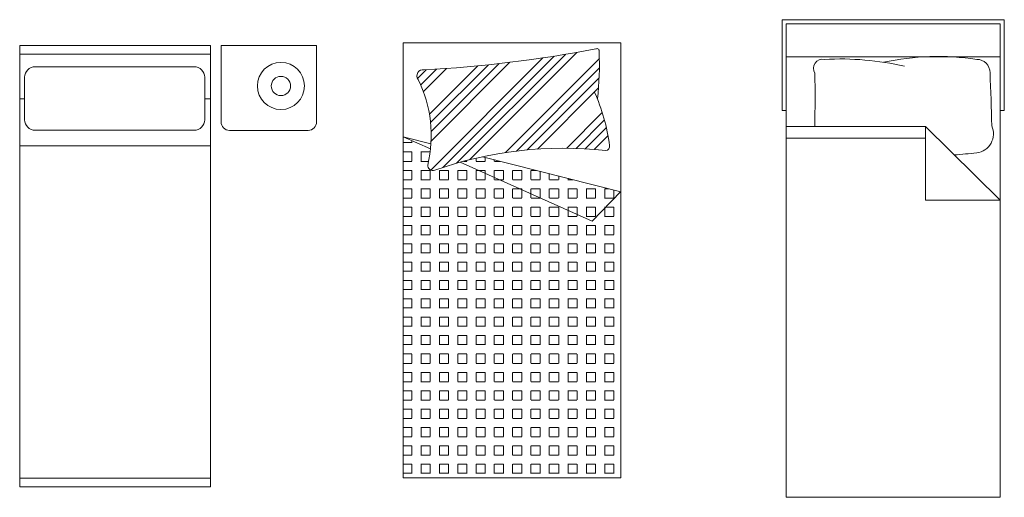
# Model space of a CAD drawing. Units: inches. Extents: x 1994 to 3075, y 3517 to 3950.
# Tile 4 of 58: x 1993.9156 to 1994.0985, y 3553.425 to 3553.5137. Entities that reach past the tile are written whole.
import ezdxf

# ---------------------------------------------------------------- set-up
doc = ezdxf.new("R2010")
doc.units = ezdxf.units.IN
doc.layers.add('A-FURN-REFR', color=8, linetype='Continuous', lineweight=13)
doc.layers.add('A-FURN-REFR-PATT', color=8, linetype='Continuous', lineweight=13)

msp = doc.modelspace()

# ---------------------------------------------------------------- hatches: boundary and pattern name
at = {"layer": 'A-FURN-REFR-PATT'}
h = msp.add_hatch(dxfattribs=at)
h.set_pattern_fill('ANSI34', color=256, scale=0.0003937007874016, style=0)
h.set_pattern_definition([(45, (1992.421944108623, 3552.870363246412), (-0.0053033008588991, 0.0053033008588991), []), (45, (1992.423711876339, 3552.870363246412), (-0.0053033008588991, 0.0053033008588991), []), (45, (1992.425479644056, 3552.870363246412), (-0.0053033008588991, 0.0053033008588991), []), (45, (1992.427247415709, 3552.870363246412), (-0.0053033008588991, 0.0053033008588991), [])])
h.paths.add_polyline_path([(1993.990115995337, 3553.504312261099, 0.3906811292884666), (1993.989395701099, 3553.503028519263, -0.1786183787400851), (1993.991383087467, 3553.486689302322, 0.5331944561183694), (1993.992669435749, 3553.485725398598, -0.1138350908180215), (1994.024455140842, 3553.489361875478, 0.4018271308504459), (1994.025167534964, 3553.490310392768, 0.0637529022039059), (1994.022888106701, 3553.498966425117, 0.0441980254026644), (1994.023194065573, 3553.508103659458, 0.2060157581720081), (1994.022937858968, 3553.508291233899, -0.033478375592124)])
h = msp.add_hatch(dxfattribs=at)
h.set_pattern_fill('SQUARE', color=256, scale=0.0005368647100931, style=0)
h.set_pattern_definition([(0, (1992.421944108623, 3552.870363246412), (0, 0.0017045454545455), [0.0017045454545455, -0.0017045454545455]), (90, (1992.421944108623, 3552.870363246412), (-0.0017045454545455, 0), [0.0017045454545455, -0.0017045454545455])])
h.paths.add_polyline_path([(1993.986843200924, 3553.428606654402), (1994.02722811466, 3553.428606654402), (1994.02722811466, 3553.481750477539), (1994.021907523152, 3553.476285841424), (1993.997414437724, 3553.487222591514, 0.0174826565834199), (1993.992669435749, 3553.485725398598, -0.5987234967258536), (1993.991383087467, 3553.486689302322, 0.0320212471709692), (1993.991893053683, 3553.489688021914), (1993.986843200924, 3553.491942902287)])
h.paths.add_polyline_path([(1994.00153542735, 3553.488234848997, 0.0149090101017854), (1993.997414437724, 3553.487222591514), (1994.021907523152, 3553.476285841424), (1994.02722811466, 3553.481750477539)], flags=17)

# ---------------------------------------------------------------- linework, layer by layer
at = {"layer": 'A-FURN-REFR'}
for p, q in [((1994.057231186005, 3553.496793440019), (1994.057231186005, 3553.513668440019)), ((1994.057231186005, 3553.513668440019), (1994.098481186005, 3553.513668440019)), ((1994.057981186005, 3553.51291844002), (1994.097731186004, 3553.51291844002)), ((1994.057981186005, 3553.51291844002), (1994.057981186005, 3553.496793440019)), ((1994.097731186004, 3553.51291844002), (1994.097731186004, 3553.496793440019)), ((1994.098481186005, 3553.513668440019), (1994.098481186005, 3553.496793440019)), ((1993.915581776324, 3553.426961523701), (1993.915581776324, 3553.508851287482)), ((1993.95101484719, 3553.508851287482), (1993.915581776324, 3553.508851287482)), ((1993.95101484719, 3553.426961523701), (1993.95101484719, 3553.508851287482)), ((1993.970718731013, 3553.508851287482), (1993.95300219558, 3553.508851287482)), ((1993.95300219558, 3553.508851287482), (1993.95300219558, 3553.494695899094)), ((1993.970718731013, 3553.494695899094), (1993.970718731013, 3553.508851287482)), ((1993.986843200924, 3553.509376481874), (1993.986843200924, 3553.428606654402)), ((1994.02722811466, 3553.509376481874), (1993.986843200924, 3553.509376481874)), ((1994.02722811466, 3553.509376481874), (1993.986843200924, 3553.509376481874)), ((1993.986843200924, 3553.509376481874), (1993.986843200924, 3553.428606654402)), ((1994.02722811466, 3553.493931850356), (1994.02722811466, 3553.509376481874)), ((1993.95101484719, 3553.507276484332), (1993.915581776324, 3553.507276484332)), ((1994.057981186005, 3553.425015883731), (1994.057981186005, 3553.50679344002)), ((1994.057981186005, 3553.50679344002), (1994.097731186004, 3553.50679344002)), ((1994.097731186004, 3553.50679344002), (1994.097731186004, 3553.425015883731)), ((1993.947992092256, 3553.504945443419), (1993.918464533201, 3553.504945443419)), ((1993.916496029264, 3553.502976939482), (1993.916496029264, 3553.495102923733)), ((1993.949960596193, 3553.495102923733), (1993.949960596193, 3553.502976939482)), ((1993.915581776324, 3553.498983996079), (1993.916496029264, 3553.498983996079)), ((1993.949960596193, 3553.498983996079), (1993.95101484719, 3553.498983996079)), ((1994.057981186005, 3553.496793440019), (1994.057231186005, 3553.496793440019)), ((1994.098481186005, 3553.496793440019), (1994.097731186004, 3553.496793440019)), ((1993.918464533201, 3553.493134419797), (1993.947992092256, 3553.493134419797)), ((1993.954576998729, 3553.493121095944), (1993.969143927863, 3553.493121095944)), ((1994.02722811466, 3553.428606654402), (1994.02722811466, 3553.493931850356)), ((1994.02722811466, 3553.428606654402), (1994.02722811466, 3553.493931850356)), ((1994.057982386004, 3553.49383344002), (1994.083847686004, 3553.49383344002)), ((1994.083847686004, 3553.49383344002), (1994.083847686004, 3553.48015344002)), ((1994.097732686005, 3553.48015344002), (1994.083847686004, 3553.49383344002)), ((1993.986843200924, 3553.491942902287), (1993.991974039738, 3553.490647970996)), ((1993.986843200924, 3553.491942902287), (1993.991893053683, 3553.489688021914)), ((1994.083847686004, 3553.49167344002), (1994.057982386004, 3553.49167344002)), ((1993.95101484719, 3553.490280994245), (1993.915581776324, 3553.490280994245)), ((1993.997414437724, 3553.487222591514), (1994.021907523152, 3553.476285841424)), ((1994.00153542735, 3553.488234848997), (1994.027238969916, 3553.481747737869)), ((1994.021907523152, 3553.476285841424), (1994.02722811466, 3553.481750477539)), ((1994.083847686004, 3553.48015344002), (1994.097732686005, 3553.48015344002)), ((1993.915581776324, 3553.428536326852), (1993.95101484719, 3553.428536326852)), ((1993.986843200924, 3553.428606654402), (1994.02722811466, 3553.428606654402)), ((1993.986843200924, 3553.428606654402), (1994.02722811466, 3553.428606654402)), ((1993.915581776324, 3553.426961523701), (1993.95101484719, 3553.426961523701)), ((1994.097731186004, 3553.425015883731), (1994.057981186005, 3553.425015883731))]:
    msp.add_line(p, q, dxfattribs=at)
for radius in [0.0043699566549229, 0.0017877096733892]:
    msp.add_circle((1993.96410790971, 3553.501367608838), radius, dxfattribs=at)
for centre, radius, start, end in [((1993.976847222788, 3553.751124534245), 0.2471686843034018, 273.2065735227801, 280.6724426503409), ((1994.022848001619, 3553.507899735766), 0.0004016778958181, 335.3666302606216, 124.3462873487214), ((1993.971458549436, 3553.505262275511), 0.051813483694514, 353.0207497140535, 2.732422750302244), ((1994.064754763306, 3553.50461832651), 0.0017217387327707, 78.72778623498706, 211.6094986857782), ((1994.064754763306, 3553.50461832651), 0.0017217387327707, 78.72778623498706, 211.6094986857782), ((1994.067944033029, 3553.452747150095), 0.0536356196908511, 77.05638185161688, 93.04883220562752), ((1994.067944033029, 3553.452747150095), 0.0536356196908511, 77.05638185161688, 93.04883220562752), ((1994.086179583237, 3553.458515778485), 0.0483256070365364, 81.47022635647696, 102.1032641982298), ((1994.086179583237, 3553.458515778485), 0.0483256070365364, 81.47022635647696, 102.1032641982298), ((1994.093347398263, 3553.503829268559), 0.0024775836026722, 0, 90), ((1994.093347398263, 3553.503829268559), 0.0024775836026722, 0, 90), ((1993.918464533201, 3553.502976939482), 0.0019685039370078, 90, 180), ((1993.947992092256, 3553.502976939482), 0.0019685039370078, 0, 90), ((1993.990451941527, 3553.503279819441), 0.0010857235472127, 78.25949602031199, 219.8002378080148), ((1993.885963234487, 3553.499370563669), 0.1773784605747312, 358.2111392619709, 1.403751564921032), ((1993.885963234487, 3553.499370563669), 0.1773784605747312, 358.2111392619709, 1.403751564921032), ((1993.801132748961, 3553.489240785046), 0.2950531070603349, 0.9125644663952034, 2.834064295864955), ((1993.801132748961, 3553.489240785046), 0.2950531070603349, 0.9125644663952034, 2.834064295864955), ((1993.968250124386, 3553.492166047153), 0.0237724360313167, 346.680428679662, 25.99366257463764), ((1993.990222103011, 3553.485736211543), 0.0352435291682859, 7.457332088483644, 24.3977020455474), ((1993.918464533201, 3553.495102923733), 0.0019685039370081, 180, 270), ((1993.947992092256, 3553.495102923733), 0.0019685039370081, 270, 0), ((1993.954576998729, 3553.494695899094), 0.0015748031496063, 180, 270), ((1993.969143927863, 3553.494695899094), 0.0015748031496063, 270, 0), ((1994.092913660596, 3553.492474359173), 0.0035513056944607, 277.015318444972, 24.37436785420747), ((1994.092913660596, 3553.492474359173), 0.0035513056944607, 277.015318444972, 24.37436785420747), ((1994.016445081357, 3553.418641745494), 0.0711723108929004, 83.53797831642504, 109.5152363664946), ((1994.024316495193, 3553.490207791067), 0.0008572023102928, 279.3080248288729, 8.069301309485365), ((1994.07894854812, 3553.626236027317), 0.1380394109326758, 274.2520388385357, 275.9873971424126), ((1994.07894854812, 3553.626236027317), 0.1380394109326758, 274.2520388385357, 275.9873971424126), ((1993.992349722133, 3553.486639014827), 0.0009679418419567, 177.0219708818246, 289.7372143522833)]:
    msp.add_arc(centre, radius, start, end, dxfattribs=at)

doc.saveas('drawing.dxf')
